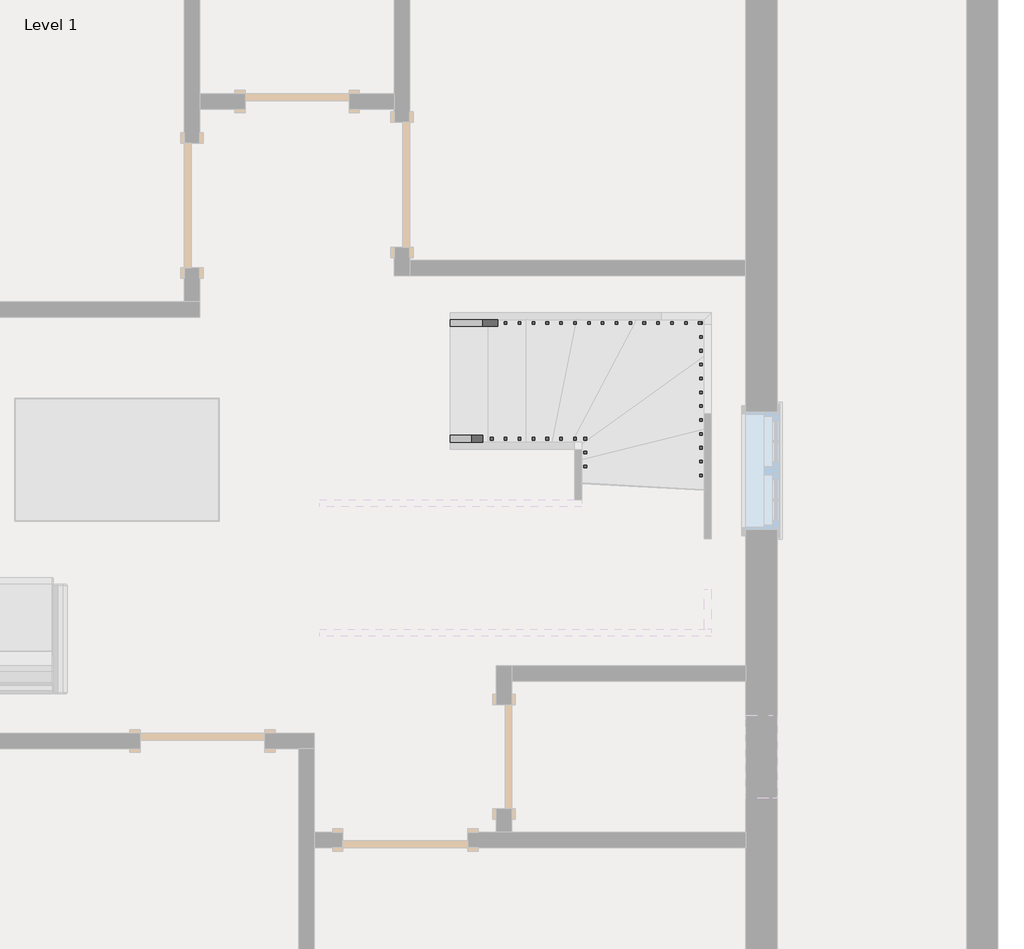
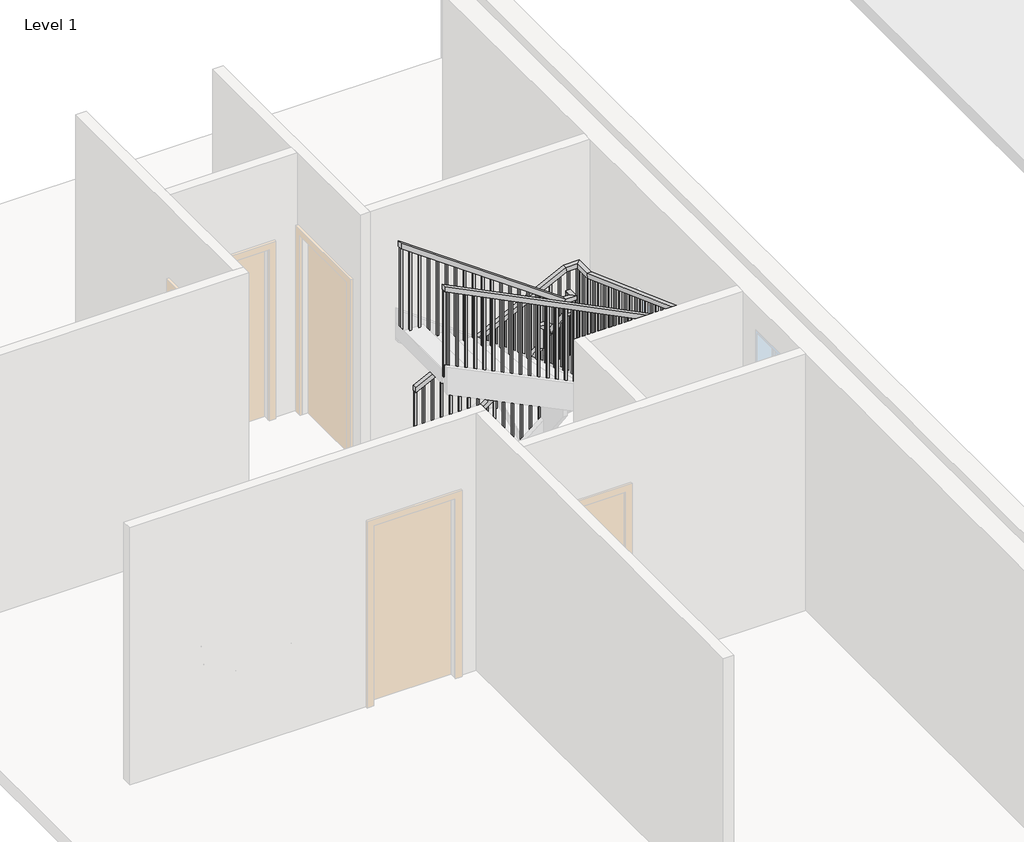
# One storey, part 2 of 3: 2 railings.
"""IFC4 building model written with IfcOpenShell, lengths in millimetres."""

from ifc_helpers import new_model, si_unit, frame, origin, place, context, project, spatial, polyline, outline, extrude, faceted_brep, element, save

model = new_model("IFC4")

# Units and contexts
model_context = context("Model", 3, world=origin())
ifc_project = project(units=[si_unit("LENGTHUNIT", "METRE", prefix="MILLI")], contexts=[model_context])

# Site, building, storey
site = spatial("IfcSite", under=ifc_project)
building = spatial("IfcBuilding", under=site)
storey = spatial("IfcBuildingStorey", under=building, Name="Level 1", Elevation=0.0)

# Railings
placement = place(None, origin())
element("IfcRailing", 1, ObjectType="Handrail - Rectangular", at=placement, inside=storey, context=model_context, shape_type="SolidModel", body=[
    faceted_brep([(158.6923968, 2074.8935985, 1083.7333333), (158.6923968, 2074.8935985, 1020.0053174), (158.6923968, 2024.0935985, 1020.0053174), (158.6923968, 2024.0935985, 1083.7333333), (1047.1901835, 2074.8935985, 1756.732376), (1097.9901835, 2074.8935985, 1731.4831856), (1097.9901835, 2024.0935985, 1731.4831856), (1047.1901835, 2024.0935985, 1756.732376), (1047.1901835, 2074.8935985, 2011.0303182), (1097.9901835, 2074.8935985, 1960.2303182), (1097.9901835, 2024.0935985, 1960.2303182), (1047.1901835, 2024.0935985, 2011.0303182), (1174.1901835, 2074.8935985, 2011.0303182), (1174.1901835, 2074.8935985, 1960.2303182), (1123.3901835, 2024.0935985, 1960.2303182), (1123.3901835, 2024.0935985, 2011.0303182), (1174.1901835, 1947.8935985, 2011.0303182), (1174.1901835, 1922.7437783, 1960.2303182), (1123.3901835, 1922.7437783, 1960.2303182), (1123.3901835, 1947.8935985, 2011.0303182), (1174.1901835, 1627.4476133, 2431.33697), (1174.1901835, 1576.6476133, 2414.1805221), (1123.3901835, 1576.6476133, 2414.1805221), (1123.3901835, 1627.4476133, 2431.33697), (1174.1901835, 1627.4476133, 2652.5821578), (1174.1901835, 1576.6476133, 2601.7821578), (1123.3901835, 1576.6476133, 2601.7821578), (1123.3901835, 1627.4476133, 2652.5821578), (1174.1901835, 1500.4476133, 2652.5821578), (1174.1901835, 1500.4476133, 2601.7821578), (1123.3901835, 1551.2476133, 2601.7821578), (1123.3901835, 1551.2476133, 2652.5821578), (1047.1901835, 1500.4476133, 2652.5821578), (1030.9951821, 1500.4476133, 2601.7821578), (1030.9951821, 1551.2476133, 2601.7821578), (1047.1901835, 1551.2476133, 2652.5821578), (-798.3242294, 1500.4476133, 3962.4), (-798.3242294, 1551.2476133, 3962.4), (-798.3242294, 1551.2476133, 3900.1059138), (-798.3242294, 1500.4476133, 3900.1059138)], [[[0, 1, 2, 3]], [[1, 0, 4, 5]], [[2, 1, 5, 6]], [[3, 2, 6, 7]], [[0, 3, 7, 4]], [[5, 4, 8, 9]], [[6, 5, 9, 10]], [[7, 6, 10, 11]], [[4, 7, 11, 8]], [[9, 8, 12, 13]], [[10, 9, 13, 14]], [[11, 10, 14, 15]], [[8, 11, 15, 12]], [[13, 12, 16, 17]], [[14, 13, 17, 18]], [[15, 14, 18, 19]], [[12, 15, 19, 16]], [[17, 16, 20, 21]], [[18, 17, 21, 22]], [[19, 18, 22, 23]], [[16, 19, 23, 20]], [[21, 20, 24, 25]], [[22, 21, 25, 26]], [[23, 22, 26, 27]], [[20, 23, 27, 24]], [[25, 24, 28, 29]], [[26, 25, 29, 30]], [[27, 26, 30, 31]], [[24, 27, 31, 28]], [[29, 28, 32, 33]], [[30, 29, 33, 34]], [[31, 30, 34, 35]], [[28, 31, 35, 32]], [[36, 37, 38, 39]], [[33, 32, 36, 39]], [[34, 33, 39, 38]], [[35, 34, 38, 37]], [[32, 35, 37, 36]]]),
    extrude(outline(polyline([(3881.4830025, -772.0848165), (3895.0033683, -791.1348165), (2878.6666667, -791.1348165), (2878.6666667, -772.0848165), (3881.4830025, -772.0848165)])), frame((0.0, 1516.3226133, 0.0), z_axis=(0.0, 1.0, 0.0), x_axis=(0.0, 0.0, 1.0)), (0.0, 0.0, 1.0), 19.05),
    extrude(outline(polyline([(3809.3743851, -670.4848165), (3822.8947509, -689.5348165), (2878.6666667, -689.5348165), (2878.6666667, -670.4848165), (3809.3743851, -670.4848165)])), frame((0.0, 1516.3226133, 0.0), z_axis=(0.0, 1.0, 0.0), x_axis=(0.0, 0.0, 1.0)), (0.0, 0.0, 1.0), 19.05),
    extrude(outline(polyline([(3737.2657677, -568.8848165), (3750.7861334, -587.9348165), (2878.6666667, -587.9348165), (2878.6666667, -568.8848165), (3737.2657677, -568.8848165)])), frame((0.0, 1516.3226133, 0.0), z_axis=(0.0, 1.0, 0.0), x_axis=(0.0, 0.0, 1.0)), (0.0, 0.0, 1.0), 19.05),
    extrude(outline(polyline([(3665.1571502, -467.2848165), (3678.677516, -486.3348165), (2709.3333333, -486.3348165), (2709.3333333, -467.2848165), (3665.1571502, -467.2848165)])), frame((0.0, 1516.3226133, 0.0), z_axis=(0.0, 1.0, 0.0), x_axis=(0.0, 0.0, 1.0)), (0.0, 0.0, 1.0), 19.05),
    extrude(outline(polyline([(3593.0485328, -365.6848165), (3606.5688986, -384.7348165), (2709.3333333, -384.7348165), (2709.3333333, -365.6848165), (3593.0485328, -365.6848165)])), frame((0.0, 1516.3226133, 0.0), z_axis=(0.0, 1.0, 0.0), x_axis=(0.0, 0.0, 1.0)), (0.0, 0.0, 1.0), 19.05),
    extrude(outline(polyline([(3520.9399154, -264.0848165), (3534.4602811, -283.1348165), (2709.3333333, -283.1348165), (2709.3333333, -264.0848165), (3520.9399154, -264.0848165)])), frame((0.0, 1516.3226133, 0.0), z_axis=(0.0, 1.0, 0.0), x_axis=(0.0, 0.0, 1.0)), (0.0, 0.0, 1.0), 19.05),
    extrude(outline(polyline([(3448.8312979, -162.4848165), (3462.3516637, -181.5348165), (2540.0, -181.5348165), (2540.0, -162.4848165), (3448.8312979, -162.4848165)])), frame((0.0, 1516.3226133, 0.0), z_axis=(0.0, 1.0, 0.0), x_axis=(0.0, 0.0, 1.0)), (0.0, 0.0, 1.0), 19.05),
    extrude(outline(polyline([(3376.7226805, -60.8848165), (3390.2430462, -79.9348165), (2540.0, -79.9348165), (2540.0, -60.8848165), (3376.7226805, -60.8848165)])), frame((0.0, 1516.3226133, 0.0), z_axis=(0.0, 1.0, 0.0), x_axis=(0.0, 0.0, 1.0)), (0.0, 0.0, 1.0), 19.05),
    extrude(outline(polyline([(3304.614063, 40.7151835), (3318.1344288, 21.6651835), (2370.6666667, 21.6651835), (2370.6666667, 40.7151835), (3304.614063, 40.7151835)])), frame((0.0, 1516.3226133, 0.0), z_axis=(0.0, 1.0, 0.0), x_axis=(0.0, 0.0, 1.0)), (0.0, 0.0, 1.0), 19.05),
    extrude(outline(polyline([(3232.5054456, 142.3151835), (3246.0258114, 123.2651835), (2370.6666667, 123.2651835), (2370.6666667, 142.3151835), (3232.5054456, 142.3151835)])), frame((0.0, 1516.3226133, 0.0), z_axis=(0.0, 1.0, 0.0), x_axis=(0.0, 0.0, 1.0)), (0.0, 0.0, 1.0), 19.05),
    extrude(outline(polyline([(3160.3968282, 243.9151835), (3173.9171939, 224.8651835), (2370.6666667, 224.8651835), (2370.6666667, 243.9151835), (3160.3968282, 243.9151835)])), frame((0.0, 1516.3226133, 0.0), z_axis=(0.0, 1.0, 0.0), x_axis=(0.0, 0.0, 1.0)), (0.0, 0.0, 1.0), 19.05),
    extrude(outline(polyline([(3088.2882107, 345.5151835), (3101.8085765, 326.4651835), (2201.3333333, 326.4651835), (2201.3333333, 345.5151835), (3088.2882107, 345.5151835)])), frame((0.0, 1516.3226133, 0.0), z_axis=(0.0, 1.0, 0.0), x_axis=(0.0, 0.0, 1.0)), (0.0, 0.0, 1.0), 19.05),
    extrude(outline(polyline([(3016.1795933, 447.1151835), (3029.6999591, 428.0651835), (2201.3333333, 428.0651835), (2201.3333333, 447.1151835), (3016.1795933, 447.1151835)])), frame((0.0, 1516.3226133, 0.0), z_axis=(0.0, 1.0, 0.0), x_axis=(0.0, 0.0, 1.0)), (0.0, 0.0, 1.0), 19.05),
    extrude(outline(polyline([(2944.0709758, 548.7151835), (2957.5913416, 529.6651835), (2032.0, 529.6651835), (2032.0, 548.7151835), (2944.0709758, 548.7151835)])), frame((0.0, 1516.3226133, 0.0), z_axis=(0.0, 1.0, 0.0), x_axis=(0.0, 0.0, 1.0)), (0.0, 0.0, 1.0), 19.05),
    extrude(outline(polyline([(2871.9623584, 650.3151835), (2885.4827242, 631.2651835), (2032.0, 631.2651835), (2032.0, 650.3151835), (2871.9623584, 650.3151835)])), frame((0.0, 1516.3226133, 0.0), z_axis=(0.0, 1.0, 0.0), x_axis=(0.0, 0.0, 1.0)), (0.0, 0.0, 1.0), 19.05),
    extrude(outline(polyline([(2799.853741, 751.9151835), (2813.3741067, 732.8651835), (2032.0, 732.8651835), (2032.0, 751.9151835), (2799.853741, 751.9151835)])), frame((0.0, 1516.3226133, 0.0), z_axis=(0.0, 1.0, 0.0), x_axis=(0.0, 0.0, 1.0)), (0.0, 0.0, 1.0), 19.05),
    extrude(outline(polyline([(2727.7451235, 853.5151835), (2741.2654893, 834.4651835), (1862.6666667, 834.4651835), (1862.6666667, 853.5151835), (2727.7451235, 853.5151835)])), frame((0.0, 1516.3226133, 0.0), z_axis=(0.0, 1.0, 0.0), x_axis=(0.0, 0.0, 1.0)), (0.0, 0.0, 1.0), 19.05),
    extrude(outline(polyline([(2655.6365061, 955.1151835), (2669.1568719, 936.0651835), (1862.6666667, 936.0651835), (1862.6666667, 955.1151835), (2655.6365061, 955.1151835)])), frame((0.0, 1516.3226133, 0.0), z_axis=(0.0, 1.0, 0.0), x_axis=(0.0, 0.0, 1.0)), (0.0, 0.0, 1.0), 19.05),
    extrude(outline(polyline([(2583.5278887, 1056.7151835), (2597.0482544, 1037.6651835), (1693.3333333, 1037.6651835), (1693.3333333, 1056.7151835), (2583.5278887, 1056.7151835)])), frame((0.0, 1516.3226133, 0.0), z_axis=(0.0, 1.0, 0.0), x_axis=(0.0, 0.0, 1.0)), (0.0, 0.0, 1.0), 19.05),
    extrude(outline(polyline([(1139.2651835, 1551.0185985), (1158.3151835, 1551.0185985), (1158.3151835, 1531.9685985), (1139.2651835, 1531.9685985), (1139.2651835, 1551.0185985)])), frame((0.0, 0.0, 1524.0), z_axis=(0.0, 0.0, 1.0), x_axis=(1.0, 0.0, 0.0)), (0.0, 0.0, 1.0), 1077.7821578),
    extrude(outline(polyline([(1633.5685985, 2339.5212353), (1652.6185985, 2314.5346787), (1652.6185985, 1354.6666667), (1633.5685985, 1354.6666667), (1633.5685985, 2339.5212353)])), frame((1139.2651835, 0.0, 0.0), z_axis=(1.0, 0.0, 0.0), x_axis=(0.0, 1.0, 0.0)), (0.0, 0.0, 1.0), 19.05),
    extrude(outline(polyline([(1735.1685985, 2206.2596006), (1754.2185985, 2181.273044), (1754.2185985, 1354.6666667), (1735.1685985, 1354.6666667), (1735.1685985, 2206.2596006)])), frame((1139.2651835, 0.0, 0.0), z_axis=(1.0, 0.0, 0.0), x_axis=(0.0, 1.0, 0.0)), (0.0, 0.0, 1.0), 19.05),
    extrude(outline(polyline([(1836.7685985, 2072.9979659), (1855.8185985, 2048.0114093), (1855.8185985, 1185.3333333), (1836.7685985, 1185.3333333), (1836.7685985, 2072.9979659)])), frame((1139.2651835, 0.0, 0.0), z_axis=(1.0, 0.0, 0.0), x_axis=(0.0, 1.0, 0.0)), (0.0, 0.0, 1.0), 19.05),
    extrude(outline(polyline([(1938.3685985, 1939.7363312), (1957.4185985, 1914.7497746), (1957.4185985, 1016.0), (1938.3685985, 1016.0), (1938.3685985, 1939.7363312)])), frame((1139.2651835, 0.0, 0.0), z_axis=(1.0, 0.0, 0.0), x_axis=(0.0, 1.0, 0.0)), (0.0, 0.0, 1.0), 19.05),
    extrude(outline(polyline([(1063.5673968, 2039.9685985), (1063.5673968, 2059.0185985), (1082.6173968, 2059.0185985), (1082.6173968, 2039.9685985), (1063.5673968, 2039.9685985)])), frame((0.0, 0.0, 846.6666667), z_axis=(0.0, 0.0, 1.0), x_axis=(1.0, 0.0, 0.0)), (0.0, 0.0, 1.0), 1113.5636515),
    extrude(outline(polyline([(1642.8813066, 981.0173968), (1628.451747, 961.9673968), (677.3333333, 961.9673968), (677.3333333, 981.0173968), (1642.8813066, 981.0173968)])), frame((0.0, 2039.9685985, 0.0), z_axis=(0.0, 1.0, 0.0), x_axis=(0.0, 0.0, 1.0)), (0.0, 0.0, 1.0), 19.05),
    extrude(outline(polyline([(1565.9236554, 879.4173968), (1551.4940958, 860.3673968), (508.0, 860.3673968), (508.0, 879.4173968), (1565.9236554, 879.4173968)])), frame((0.0, 2039.9685985, 0.0), z_axis=(0.0, 1.0, 0.0), x_axis=(0.0, 0.0, 1.0)), (0.0, 0.0, 1.0), 19.05),
    extrude(outline(polyline([(1488.9660042, 777.8173968), (1474.5364446, 758.7673968), (508.0, 758.7673968), (508.0, 777.8173968), (1488.9660042, 777.8173968)])), frame((0.0, 2039.9685985, 0.0), z_axis=(0.0, 1.0, 0.0), x_axis=(0.0, 0.0, 1.0)), (0.0, 0.0, 1.0), 19.05),
    extrude(outline(polyline([(1412.008353, 676.2173968), (1397.5787934, 657.1673968), (338.6666667, 657.1673968), (338.6666667, 676.2173968), (1412.008353, 676.2173968)])), frame((0.0, 2039.9685985, 0.0), z_axis=(0.0, 1.0, 0.0), x_axis=(0.0, 0.0, 1.0)), (0.0, 0.0, 1.0), 19.05),
    extrude(outline(polyline([(1335.0507019, 574.6173968), (1320.6211423, 555.5673968), (338.6666667, 555.5673968), (338.6666667, 574.6173968), (1335.0507019, 574.6173968)])), frame((0.0, 2039.9685985, 0.0), z_axis=(0.0, 1.0, 0.0), x_axis=(0.0, 0.0, 1.0)), (0.0, 0.0, 1.0), 19.05),
    extrude(outline(polyline([(1258.0930507, 473.0173968), (1243.6634911, 453.9673968), (338.6666667, 453.9673968), (338.6666667, 473.0173968), (1258.0930507, 473.0173968)])), frame((0.0, 2039.9685985, 0.0), z_axis=(0.0, 1.0, 0.0), x_axis=(0.0, 0.0, 1.0)), (0.0, 0.0, 1.0), 19.05),
    extrude(outline(polyline([(1181.1353995, 371.4173968), (1166.7058399, 352.3673968), (169.3333333, 352.3673968), (169.3333333, 371.4173968), (1181.1353995, 371.4173968)])), frame((0.0, 2039.9685985, 0.0), z_axis=(0.0, 1.0, 0.0), x_axis=(0.0, 0.0, 1.0)), (0.0, 0.0, 1.0), 19.05),
    extrude(outline(polyline([(1104.1777483, 269.8173968), (1089.7481887, 250.7673968), (169.3333333, 250.7673968), (169.3333333, 269.8173968), (1104.1777483, 269.8173968)])), frame((0.0, 2039.9685985, 0.0), z_axis=(0.0, 1.0, 0.0), x_axis=(0.0, 0.0, 1.0)), (0.0, 0.0, 1.0), 19.05),
    extrude(outline(polyline([(1139.2651835, 1535.3726133), (1158.3151835, 1535.3726133), (1158.3151835, 1516.3226133), (1139.2651835, 1516.3226133), (1139.2651835, 1535.3726133)])), frame((0.0, 0.0, 1524.0), z_axis=(0.0, 0.0, 1.0), x_axis=(1.0, 0.0, 0.0)), (0.0, 0.0, 1.0), 1077.7821578),
    extrude(outline(polyline([(1139.2651835, 2039.9685985), (1139.2651835, 2059.0185985), (1158.3151835, 2059.0185985), (1158.3151835, 2039.9685985), (1139.2651835, 2039.9685985)])), frame((0.0, 0.0, 846.6666667), z_axis=(0.0, 0.0, 1.0), x_axis=(1.0, 0.0, 0.0)), (0.0, 0.0, 1.0), 1113.5636515),
    extrude(outline(polyline([(3886.585548, -779.2742294), (3900.1059138, -798.3242294), (2878.6666667, -798.3242294), (2878.6666667, -779.2742294), (3886.585548, -779.2742294)])), frame((0.0, 1516.3226133, 0.0), z_axis=(0.0, 1.0, 0.0), x_axis=(0.0, 0.0, 1.0)), (0.0, 0.0, 1.0), 19.05),
    extrude(outline(polyline([(1034.434877, 177.7423968), (1020.0053174, 158.6923968), (169.3333333, 158.6923968), (169.3333333, 177.7423968), (1034.434877, 177.7423968)])), frame((0.0, 2039.9685985, 0.0), z_axis=(0.0, 1.0, 0.0), x_axis=(0.0, 0.0, 1.0)), (0.0, 0.0, 1.0), 19.05),
])
element("IfcRailing", 2, ObjectType="Handrail - Rectangular", at=placement, inside=storey, context=model_context, shape_type="SolidModel", body=[
    faceted_brep([(158.6923968, 2922.8476133, 1083.7333333), (158.6923968, 2922.8476133, 1027.0325724), (158.6923968, 2872.0476133, 1027.0325724), (158.6923968, 2872.0476133, 1083.7333333), (1841.0143863, 2922.8476133, 1917.8084972), (1852.9161672, 2922.8476133, 1867.0084972), (1852.9161672, 2872.0476133, 1867.0084972), (1841.0143863, 2872.0476133, 1917.8084972), (2022.1441983, 2922.8476133, 1917.8084972), (2022.1441983, 2922.8476133, 1867.0084972), (1971.3441983, 2872.0476133, 1867.0084972), (1971.3441983, 2872.0476133, 1917.8084972), (2022.1441983, 2686.7050655, 1917.8084972), (2022.1441983, 2677.692274, 1867.0084972), (1971.3441983, 2677.692274, 1867.0084972), (1971.3441983, 2686.7050655, 1917.8084972), (2022.1441983, 796.951655, 2610.1505936), (2022.1441983, 787.9388635, 2559.3505936), (1971.3441983, 787.9388635, 2559.3505936), (1971.3441983, 796.951655, 2610.1505936), (2022.1441983, 652.4935985, 2610.1505936), (2022.1441983, 652.4935985, 2559.3505936), (1971.3441983, 703.2935985, 2559.3505936), (1971.3441983, 703.2935985, 2610.1505936), (1909.402346, 652.4935985, 2610.1505936), (1897.4228813, 652.4935985, 2559.3505936), (1897.4228813, 703.2935985, 2559.3505936), (1909.402346, 703.2935985, 2610.1505936), (-798.3242294, 652.4935985, 3962.4), (-798.3242294, 703.2935985, 3962.4), (-798.3242294, 703.2935985, 3905.6174077), (-798.3242294, 652.4935985, 3905.6174077)], [[[0, 1, 2, 3]], [[1, 0, 4, 5]], [[2, 1, 5, 6]], [[3, 2, 6, 7]], [[0, 3, 7, 4]], [[5, 4, 8, 9]], [[6, 5, 9, 10]], [[7, 6, 10, 11]], [[4, 7, 11, 8]], [[9, 8, 12, 13]], [[10, 9, 13, 14]], [[11, 10, 14, 15]], [[8, 11, 15, 12]], [[13, 12, 16, 17]], [[14, 13, 17, 18]], [[15, 14, 18, 19]], [[12, 15, 19, 16]], [[17, 16, 20, 21]], [[18, 17, 21, 22]], [[19, 18, 22, 23]], [[16, 19, 23, 20]], [[21, 20, 24, 25]], [[22, 21, 25, 26]], [[23, 22, 26, 27]], [[20, 23, 27, 24]], [[28, 29, 30, 31]], [[25, 24, 28, 31]], [[26, 25, 31, 30]], [[27, 26, 30, 29]], [[24, 27, 29, 28]]]),
    extrude(outline(polyline([(3884.4709318, -755.9808017), (2878.6666667, -755.9808017), (2878.6666667, -736.9308017), (3874.9572862, -736.9308017), (3884.4709318, -755.9808017)])), frame((0.0, 668.3685985, 0.0), z_axis=(0.0, 1.0, 0.0), x_axis=(0.0, 0.0, 1.0)), (0.0, 0.0, 1.0), 19.05),
    extrude(outline(polyline([(3833.7314883, -654.3808017), (2878.6666667, -654.3808017), (2878.6666667, -635.3308017), (3824.2178426, -635.3308017), (3833.7314883, -654.3808017)])), frame((0.0, 668.3685985, 0.0), z_axis=(0.0, 1.0, 0.0), x_axis=(0.0, 0.0, 1.0)), (0.0, 0.0, 1.0), 19.05),
    extrude(outline(polyline([(3782.9920447, -552.7808017), (2878.6666667, -552.7808017), (2878.6666667, -533.7308017), (3773.4783991, -533.7308017), (3782.9920447, -552.7808017)])), frame((0.0, 668.3685985, 0.0), z_axis=(0.0, 1.0, 0.0), x_axis=(0.0, 0.0, 1.0)), (0.0, 0.0, 1.0), 19.05),
    extrude(outline(polyline([(3732.2526012, -451.1808017), (2709.3333333, -451.1808017), (2709.3333333, -432.1308017), (3722.7389555, -432.1308017), (3732.2526012, -451.1808017)])), frame((0.0, 668.3685985, 0.0), z_axis=(0.0, 1.0, 0.0), x_axis=(0.0, 0.0, 1.0)), (0.0, 0.0, 1.0), 19.05),
    extrude(outline(polyline([(3681.5131577, -349.5808017), (2709.3333333, -349.5808017), (2709.3333333, -330.5308017), (3671.999512, -330.5308017), (3681.5131577, -349.5808017)])), frame((0.0, 668.3685985, 0.0), z_axis=(0.0, 1.0, 0.0), x_axis=(0.0, 0.0, 1.0)), (0.0, 0.0, 1.0), 19.05),
    extrude(outline(polyline([(3630.7737141, -247.9808017), (2540.0, -247.9808017), (2540.0, -228.9308017), (3621.2600685, -228.9308017), (3630.7737141, -247.9808017)])), frame((0.0, 668.3685985, 0.0), z_axis=(0.0, 1.0, 0.0), x_axis=(0.0, 0.0, 1.0)), (0.0, 0.0, 1.0), 19.05),
    extrude(outline(polyline([(3580.0342706, -146.3808017), (2540.0, -146.3808017), (2540.0, -127.3308017), (3570.5206249, -127.3308017), (3580.0342706, -146.3808017)])), frame((0.0, 668.3685985, 0.0), z_axis=(0.0, 1.0, 0.0), x_axis=(0.0, 0.0, 1.0)), (0.0, 0.0, 1.0), 19.05),
    extrude(outline(polyline([(3529.294827, -44.7808017), (2540.0, -44.7808017), (2540.0, -25.7308017), (3519.7811814, -25.7308017), (3529.294827, -44.7808017)])), frame((0.0, 668.3685985, 0.0), z_axis=(0.0, 1.0, 0.0), x_axis=(0.0, 0.0, 1.0)), (0.0, 0.0, 1.0), 19.05),
    extrude(outline(polyline([(3478.5553835, 56.8191983), (2370.6666667, 56.8191983), (2370.6666667, 75.8691983), (3469.0417378, 75.8691983), (3478.5553835, 56.8191983)])), frame((0.0, 668.3685985, 0.0), z_axis=(0.0, 1.0, 0.0), x_axis=(0.0, 0.0, 1.0)), (0.0, 0.0, 1.0), 19.05),
    extrude(outline(polyline([(3427.81594, 158.4191983), (2370.6666667, 158.4191983), (2370.6666667, 177.4691983), (3418.3022943, 177.4691983), (3427.81594, 158.4191983)])), frame((0.0, 668.3685985, 0.0), z_axis=(0.0, 1.0, 0.0), x_axis=(0.0, 0.0, 1.0)), (0.0, 0.0, 1.0), 19.05),
    extrude(outline(polyline([(3377.0764964, 260.0191983), (2370.6666667, 260.0191983), (2370.6666667, 279.0691983), (3367.5628508, 279.0691983), (3377.0764964, 260.0191983)])), frame((0.0, 668.3685985, 0.0), z_axis=(0.0, 1.0, 0.0), x_axis=(0.0, 0.0, 1.0)), (0.0, 0.0, 1.0), 19.05),
    extrude(outline(polyline([(3326.3370529, 361.6191983), (2201.3333333, 361.6191983), (2201.3333333, 380.6691983), (3316.8234072, 380.6691983), (3326.3370529, 361.6191983)])), frame((0.0, 668.3685985, 0.0), z_axis=(0.0, 1.0, 0.0), x_axis=(0.0, 0.0, 1.0)), (0.0, 0.0, 1.0), 19.05),
    extrude(outline(polyline([(3275.5976093, 463.2191983), (2201.3333333, 463.2191983), (2201.3333333, 482.2691983), (3266.0839637, 482.2691983), (3275.5976093, 463.2191983)])), frame((0.0, 668.3685985, 0.0), z_axis=(0.0, 1.0, 0.0), x_axis=(0.0, 0.0, 1.0)), (0.0, 0.0, 1.0), 19.05),
    extrude(outline(polyline([(3224.8581658, 564.8191983), (2201.3333333, 564.8191983), (2201.3333333, 583.8691983), (3215.3445201, 583.8691983), (3224.8581658, 564.8191983)])), frame((0.0, 668.3685985, 0.0), z_axis=(0.0, 1.0, 0.0), x_axis=(0.0, 0.0, 1.0)), (0.0, 0.0, 1.0), 19.05),
    extrude(outline(polyline([(3174.1187223, 666.4191983), (2032.0, 666.4191983), (2032.0, 685.4691983), (3164.6050766, 685.4691983), (3174.1187223, 666.4191983)])), frame((0.0, 668.3685985, 0.0), z_axis=(0.0, 1.0, 0.0), x_axis=(0.0, 0.0, 1.0)), (0.0, 0.0, 1.0), 19.05),
    extrude(outline(polyline([(3123.3792787, 768.0191983), (2032.0, 768.0191983), (2032.0, 787.0691983), (3113.865633, 787.0691983), (3123.3792787, 768.0191983)])), frame((0.0, 668.3685985, 0.0), z_axis=(0.0, 1.0, 0.0), x_axis=(0.0, 0.0, 1.0)), (0.0, 0.0, 1.0), 19.05),
    extrude(outline(polyline([(3072.6398352, 869.6191983), (2032.0, 869.6191983), (2032.0, 888.6691983), (3063.1261895, 888.6691983), (3072.6398352, 869.6191983)])), frame((0.0, 668.3685985, 0.0), z_axis=(0.0, 1.0, 0.0), x_axis=(0.0, 0.0, 1.0)), (0.0, 0.0, 1.0), 19.05),
    extrude(outline(polyline([(3021.9003916, 971.2191983), (2032.0, 971.2191983), (2032.0, 990.2691983), (3012.386746, 990.2691983), (3021.9003916, 971.2191983)])), frame((0.0, 668.3685985, 0.0), z_axis=(0.0, 1.0, 0.0), x_axis=(0.0, 0.0, 1.0)), (0.0, 0.0, 1.0), 19.05),
    extrude(outline(polyline([(2971.1609481, 1072.8191983), (1862.6666667, 1072.8191983), (1862.6666667, 1091.8691983), (2961.6473024, 1091.8691983), (2971.1609481, 1072.8191983)])), frame((0.0, 668.3685985, 0.0), z_axis=(0.0, 1.0, 0.0), x_axis=(0.0, 0.0, 1.0)), (0.0, 0.0, 1.0), 19.05),
    extrude(outline(polyline([(2920.4215046, 1174.4191983), (1862.6666667, 1174.4191983), (1862.6666667, 1193.4691983), (2910.9078589, 1193.4691983), (2920.4215046, 1174.4191983)])), frame((0.0, 668.3685985, 0.0), z_axis=(0.0, 1.0, 0.0), x_axis=(0.0, 0.0, 1.0)), (0.0, 0.0, 1.0), 19.05),
    extrude(outline(polyline([(2869.682061, 1276.0191983), (1862.6666667, 1276.0191983), (1862.6666667, 1295.0691983), (2860.1684153, 1295.0691983), (2869.682061, 1276.0191983)])), frame((0.0, 668.3685985, 0.0), z_axis=(0.0, 1.0, 0.0), x_axis=(0.0, 0.0, 1.0)), (0.0, 0.0, 1.0), 19.05),
    extrude(outline(polyline([(2818.9426175, 1377.6191983), (1693.3333333, 1377.6191983), (1693.3333333, 1396.6691983), (2809.4289718, 1396.6691983), (2818.9426175, 1377.6191983)])), frame((0.0, 668.3685985, 0.0), z_axis=(0.0, 1.0, 0.0), x_axis=(0.0, 0.0, 1.0)), (0.0, 0.0, 1.0), 19.05),
    extrude(outline(polyline([(2768.2031739, 1479.2191983), (1693.3333333, 1479.2191983), (1693.3333333, 1498.2691983), (2758.6895283, 1498.2691983), (2768.2031739, 1479.2191983)])), frame((0.0, 668.3685985, 0.0), z_axis=(0.0, 1.0, 0.0), x_axis=(0.0, 0.0, 1.0)), (0.0, 0.0, 1.0), 19.05),
    extrude(outline(polyline([(2717.4637304, 1580.8191983), (1693.3333333, 1580.8191983), (1693.3333333, 1599.8691983), (2707.9500847, 1599.8691983), (2717.4637304, 1580.8191983)])), frame((0.0, 668.3685985, 0.0), z_axis=(0.0, 1.0, 0.0), x_axis=(0.0, 0.0, 1.0)), (0.0, 0.0, 1.0), 19.05),
    extrude(outline(polyline([(2666.7242869, 1682.4191983), (1693.3333333, 1682.4191983), (1693.3333333, 1701.4691983), (2657.2106412, 1701.4691983), (2666.7242869, 1682.4191983)])), frame((0.0, 668.3685985, 0.0), z_axis=(0.0, 1.0, 0.0), x_axis=(0.0, 0.0, 1.0)), (0.0, 0.0, 1.0), 19.05),
    extrude(outline(polyline([(2615.9848433, 1784.0191983), (1693.3333333, 1784.0191983), (1693.3333333, 1803.0691983), (2606.4711976, 1803.0691983), (2615.9848433, 1784.0191983)])), frame((0.0, 668.3685985, 0.0), z_axis=(0.0, 1.0, 0.0), x_axis=(0.0, 0.0, 1.0)), (0.0, 0.0, 1.0), 19.05),
    extrude(outline(polyline([(2565.2453998, 1885.6191983), (1524.0, 1885.6191983), (1524.0, 1904.6691983), (2555.7317541, 1904.6691983), (2565.2453998, 1885.6191983)])), frame((0.0, 668.3685985, 0.0), z_axis=(0.0, 1.0, 0.0), x_axis=(0.0, 0.0, 1.0)), (0.0, 0.0, 1.0), 19.05),
    extrude(outline(polyline([(2006.2691983, 773.3726133), (2006.2691983, 754.3226133), (1987.2191983, 754.3226133), (1987.2191983, 773.3726133), (2006.2691983, 773.3726133)])), frame((0.0, 0.0, 1524.0), z_axis=(0.0, 0.0, 1.0), x_axis=(1.0, 0.0, 0.0)), (0.0, 0.0, 1.0), 1035.3505936),
    extrude(outline(polyline([(874.9726133, 2527.4643546), (874.9726133, 1524.0), (855.9226133, 1524.0), (855.9226133, 2534.443634), (874.9726133, 2527.4643546)])), frame((1987.2191983, 0.0, 0.0), z_axis=(1.0, 0.0, 0.0), x_axis=(0.0, 1.0, 0.0)), (0.0, 0.0, 1.0), 19.05),
    extrude(outline(polyline([(976.5726133, 2490.2415315), (976.5726133, 1524.0), (957.5226133, 1524.0), (957.5226133, 2497.2208108), (976.5726133, 2490.2415315)])), frame((1987.2191983, 0.0, 0.0), z_axis=(1.0, 0.0, 0.0), x_axis=(0.0, 1.0, 0.0)), (0.0, 0.0, 1.0), 19.05),
    extrude(outline(polyline([(1078.1726133, 2453.0187083), (1078.1726133, 1524.0), (1059.1226133, 1524.0), (1059.1226133, 2459.9979877), (1078.1726133, 2453.0187083)])), frame((1987.2191983, 0.0, 0.0), z_axis=(1.0, 0.0, 0.0), x_axis=(0.0, 1.0, 0.0)), (0.0, 0.0, 1.0), 19.05),
    extrude(outline(polyline([(1179.7726133, 2415.7958852), (1179.7726133, 1524.0), (1160.7226133, 1524.0), (1160.7226133, 2422.7751645), (1179.7726133, 2415.7958852)])), frame((1987.2191983, 0.0, 0.0), z_axis=(1.0, 0.0, 0.0), x_axis=(0.0, 1.0, 0.0)), (0.0, 0.0, 1.0), 19.05),
    extrude(outline(polyline([(1281.3726133, 2378.573062), (1281.3726133, 1524.0), (1262.3226133, 1524.0), (1262.3226133, 2385.5523414), (1281.3726133, 2378.573062)])), frame((1987.2191983, 0.0, 0.0), z_axis=(1.0, 0.0, 0.0), x_axis=(0.0, 1.0, 0.0)), (0.0, 0.0, 1.0), 19.05),
    extrude(outline(polyline([(1382.9726133, 2341.3502389), (1382.9726133, 1354.6666667), (1363.9226133, 1354.6666667), (1363.9226133, 2348.3295182), (1382.9726133, 2341.3502389)])), frame((1987.2191983, 0.0, 0.0), z_axis=(1.0, 0.0, 0.0), x_axis=(0.0, 1.0, 0.0)), (0.0, 0.0, 1.0), 19.05),
    extrude(outline(polyline([(1484.5726133, 2304.1274157), (1484.5726133, 1354.6666667), (1465.5226133, 1354.6666667), (1465.5226133, 2311.1066951), (1484.5726133, 2304.1274157)])), frame((1987.2191983, 0.0, 0.0), z_axis=(1.0, 0.0, 0.0), x_axis=(0.0, 1.0, 0.0)), (0.0, 0.0, 1.0), 19.05),
    extrude(outline(polyline([(1586.1726133, 2266.9045926), (1586.1726133, 1354.6666667), (1567.1226133, 1354.6666667), (1567.1226133, 2273.8838719), (1586.1726133, 2266.9045926)])), frame((1987.2191983, 0.0, 0.0), z_axis=(1.0, 0.0, 0.0), x_axis=(0.0, 1.0, 0.0)), (0.0, 0.0, 1.0), 19.05),
    extrude(outline(polyline([(1687.7726133, 2229.6817694), (1687.7726133, 1354.6666667), (1668.7226133, 1354.6666667), (1668.7226133, 2236.6610488), (1687.7726133, 2229.6817694)])), frame((1987.2191983, 0.0, 0.0), z_axis=(1.0, 0.0, 0.0), x_axis=(0.0, 1.0, 0.0)), (0.0, 0.0, 1.0), 19.05),
    extrude(outline(polyline([(1789.3726133, 2192.4589463), (1789.3726133, 1185.3333333), (1770.3226133, 1185.3333333), (1770.3226133, 2199.4382256), (1789.3726133, 2192.4589463)])), frame((1987.2191983, 0.0, 0.0), z_axis=(1.0, 0.0, 0.0), x_axis=(0.0, 1.0, 0.0)), (0.0, 0.0, 1.0), 19.05),
    extrude(outline(polyline([(1890.9726133, 2155.2361231), (1890.9726133, 1185.3333333), (1871.9226133, 1185.3333333), (1871.9226133, 2162.2154025), (1890.9726133, 2155.2361231)])), frame((1987.2191983, 0.0, 0.0), z_axis=(1.0, 0.0, 0.0), x_axis=(0.0, 1.0, 0.0)), (0.0, 0.0, 1.0), 19.05),
    extrude(outline(polyline([(1992.5726133, 2118.0133), (1992.5726133, 1185.3333333), (1973.5226133, 1185.3333333), (1973.5226133, 2124.9925793), (1992.5726133, 2118.0133)])), frame((1987.2191983, 0.0, 0.0), z_axis=(1.0, 0.0, 0.0), x_axis=(0.0, 1.0, 0.0)), (0.0, 0.0, 1.0), 19.05),
    extrude(outline(polyline([(2094.1726133, 2080.7904769), (2094.1726133, 1185.3333333), (2075.1226133, 1185.3333333), (2075.1226133, 2087.7697562), (2094.1726133, 2080.7904769)])), frame((1987.2191983, 0.0, 0.0), z_axis=(1.0, 0.0, 0.0), x_axis=(0.0, 1.0, 0.0)), (0.0, 0.0, 1.0), 19.05),
    extrude(outline(polyline([(2195.7726133, 2043.5676537), (2195.7726133, 1016.0), (2176.7226133, 1016.0), (2176.7226133, 2050.546933), (2195.7726133, 2043.5676537)])), frame((1987.2191983, 0.0, 0.0), z_axis=(1.0, 0.0, 0.0), x_axis=(0.0, 1.0, 0.0)), (0.0, 0.0, 1.0), 19.05),
    extrude(outline(polyline([(2297.3726133, 2006.3448306), (2297.3726133, 1016.0), (2278.3226133, 1016.0), (2278.3226133, 2013.3241099), (2297.3726133, 2006.3448306)])), frame((1987.2191983, 0.0, 0.0), z_axis=(1.0, 0.0, 0.0), x_axis=(0.0, 1.0, 0.0)), (0.0, 0.0, 1.0), 19.05),
    extrude(outline(polyline([(2398.9726133, 1969.1220074), (2398.9726133, 1016.0), (2379.9226133, 1016.0), (2379.9226133, 1976.1012867), (2398.9726133, 1969.1220074)])), frame((1987.2191983, 0.0, 0.0), z_axis=(1.0, 0.0, 0.0), x_axis=(0.0, 1.0, 0.0)), (0.0, 0.0, 1.0), 19.05),
    extrude(outline(polyline([(2500.5726133, 1931.8991843), (2500.5726133, 1016.0), (2481.5226133, 1016.0), (2481.5226133, 1938.8784636), (2500.5726133, 1931.8991843)])), frame((1987.2191983, 0.0, 0.0), z_axis=(1.0, 0.0, 0.0), x_axis=(0.0, 1.0, 0.0)), (0.0, 0.0, 1.0), 19.05),
    extrude(outline(polyline([(2602.1726133, 1894.6763611), (2602.1726133, 1016.0), (2583.1226133, 1016.0), (2583.1226133, 1901.6556405), (2602.1726133, 1894.6763611)])), frame((1987.2191983, 0.0, 0.0), z_axis=(1.0, 0.0, 0.0), x_axis=(0.0, 1.0, 0.0)), (0.0, 0.0, 1.0), 19.05),
    extrude(outline(polyline([(2006.2691983, 2703.7726133), (2006.2691983, 2684.7226133), (1987.2191983, 2684.7226133), (1987.2191983, 2703.7726133), (2006.2691983, 2703.7726133)])), frame((0.0, 0.0, 846.6666667), z_axis=(0.0, 0.0, 1.0), x_axis=(1.0, 0.0, 0.0)), (0.0, 0.0, 1.0), 1020.3418305),
    extrude(outline(polyline([(2006.2691983, 2805.3726133), (2006.2691983, 2786.3226133), (1987.2191983, 2786.3226133), (1987.2191983, 2805.3726133), (2006.2691983, 2805.3726133)])), frame((0.0, 0.0, 846.6666667), z_axis=(0.0, 0.0, 1.0), x_axis=(1.0, 0.0, 0.0)), (0.0, 0.0, 1.0), 1020.3418305),
    extrude(outline(polyline([(1977.9673968, 2906.9726133), (1997.0173968, 2906.9726133), (1997.0173968, 2887.9226133), (1977.9673968, 2887.9226133), (1977.9673968, 2906.9726133)])), frame((0.0, 0.0, 846.6666667), z_axis=(0.0, 0.0, 1.0), x_axis=(1.0, 0.0, 0.0)), (0.0, 0.0, 1.0), 1020.3418305),
    extrude(outline(polyline([(1876.3673968, 2906.9726133), (1895.4173968, 2906.9726133), (1895.4173968, 2887.9226133), (1876.3673968, 2887.9226133), (1876.3673968, 2906.9726133)])), frame((0.0, 0.0, 846.6666667), z_axis=(0.0, 0.0, 1.0), x_axis=(1.0, 0.0, 0.0)), (0.0, 0.0, 1.0), 1020.3418305),
    extrude(outline(polyline([(1828.2632695, 1774.7673968), (846.6666667, 1774.7673968), (846.6666667, 1793.8173968), (1837.7080321, 1793.8173968), (1828.2632695, 1774.7673968)])), frame((0.0, 2887.9226133, 0.0), z_axis=(0.0, 1.0, 0.0), x_axis=(0.0, 0.0, 1.0)), (0.0, 0.0, 1.0), 19.05),
    extrude(outline(polyline([(1777.8912021, 1673.1673968), (846.6666667, 1673.1673968), (846.6666667, 1692.2173968), (1787.3359647, 1692.2173968), (1777.8912021, 1673.1673968)])), frame((0.0, 2887.9226133, 0.0), z_axis=(0.0, 1.0, 0.0), x_axis=(0.0, 0.0, 1.0)), (0.0, 0.0, 1.0), 19.05),
    extrude(outline(polyline([(1727.5191347, 1571.5673968), (846.6666667, 1571.5673968), (846.6666667, 1590.6173968), (1736.9638973, 1590.6173968), (1727.5191347, 1571.5673968)])), frame((0.0, 2887.9226133, 0.0), z_axis=(0.0, 1.0, 0.0), x_axis=(0.0, 0.0, 1.0)), (0.0, 0.0, 1.0), 19.05),
    extrude(outline(polyline([(1677.1470673, 1469.9673968), (677.3333333, 1469.9673968), (677.3333333, 1489.0173968), (1686.5918299, 1489.0173968), (1677.1470673, 1469.9673968)])), frame((0.0, 2887.9226133, 0.0), z_axis=(0.0, 1.0, 0.0), x_axis=(0.0, 0.0, 1.0)), (0.0, 0.0, 1.0), 19.05),
    extrude(outline(polyline([(1626.7749999, 1368.3673968), (677.3333333, 1368.3673968), (677.3333333, 1387.4173968), (1636.2197625, 1387.4173968), (1626.7749999, 1368.3673968)])), frame((0.0, 2887.9226133, 0.0), z_axis=(0.0, 1.0, 0.0), x_axis=(0.0, 0.0, 1.0)), (0.0, 0.0, 1.0), 19.05),
    extrude(outline(polyline([(1576.4029325, 1266.7673968), (677.3333333, 1266.7673968), (677.3333333, 1285.8173968), (1585.8476951, 1285.8173968), (1576.4029325, 1266.7673968)])), frame((0.0, 2887.9226133, 0.0), z_axis=(0.0, 1.0, 0.0), x_axis=(0.0, 0.0, 1.0)), (0.0, 0.0, 1.0), 19.05),
    extrude(outline(polyline([(1526.0308651, 1165.1673968), (677.3333333, 1165.1673968), (677.3333333, 1184.2173968), (1535.4756277, 1184.2173968), (1526.0308651, 1165.1673968)])), frame((0.0, 2887.9226133, 0.0), z_axis=(0.0, 1.0, 0.0), x_axis=(0.0, 0.0, 1.0)), (0.0, 0.0, 1.0), 19.05),
    extrude(outline(polyline([(1475.6587977, 1063.5673968), (508.0, 1063.5673968), (508.0, 1082.6173968), (1485.1035603, 1082.6173968), (1475.6587977, 1063.5673968)])), frame((0.0, 2887.9226133, 0.0), z_axis=(0.0, 1.0, 0.0), x_axis=(0.0, 0.0, 1.0)), (0.0, 0.0, 1.0), 19.05),
    extrude(outline(polyline([(1425.2867303, 961.9673968), (508.0, 961.9673968), (508.0, 981.0173968), (1434.7314929, 981.0173968), (1425.2867303, 961.9673968)])), frame((0.0, 2887.9226133, 0.0), z_axis=(0.0, 1.0, 0.0), x_axis=(0.0, 0.0, 1.0)), (0.0, 0.0, 1.0), 19.05),
    extrude(outline(polyline([(1374.9146629, 860.3673968), (508.0, 860.3673968), (508.0, 879.4173968), (1384.3594255, 879.4173968), (1374.9146629, 860.3673968)])), frame((0.0, 2887.9226133, 0.0), z_axis=(0.0, 1.0, 0.0), x_axis=(0.0, 0.0, 1.0)), (0.0, 0.0, 1.0), 19.05),
    extrude(outline(polyline([(1324.5425955, 758.7673968), (508.0, 758.7673968), (508.0, 777.8173968), (1333.9873581, 777.8173968), (1324.5425955, 758.7673968)])), frame((0.0, 2887.9226133, 0.0), z_axis=(0.0, 1.0, 0.0), x_axis=(0.0, 0.0, 1.0)), (0.0, 0.0, 1.0), 19.05),
    extrude(outline(polyline([(1274.1705281, 657.1673968), (338.6666667, 657.1673968), (338.6666667, 676.2173968), (1283.6152907, 676.2173968), (1274.1705281, 657.1673968)])), frame((0.0, 2887.9226133, 0.0), z_axis=(0.0, 1.0, 0.0), x_axis=(0.0, 0.0, 1.0)), (0.0, 0.0, 1.0), 19.05),
    extrude(outline(polyline([(1223.7984607, 555.5673968), (338.6666667, 555.5673968), (338.6666667, 574.6173968), (1233.2432233, 574.6173968), (1223.7984607, 555.5673968)])), frame((0.0, 2887.9226133, 0.0), z_axis=(0.0, 1.0, 0.0), x_axis=(0.0, 0.0, 1.0)), (0.0, 0.0, 1.0), 19.05),
    extrude(outline(polyline([(1173.4263933, 453.9673968), (338.6666667, 453.9673968), (338.6666667, 473.0173968), (1182.8711559, 473.0173968), (1173.4263933, 453.9673968)])), frame((0.0, 2887.9226133, 0.0), z_axis=(0.0, 1.0, 0.0), x_axis=(0.0, 0.0, 1.0)), (0.0, 0.0, 1.0), 19.05),
    extrude(outline(polyline([(1123.0543259, 352.3673968), (169.3333333, 352.3673968), (169.3333333, 371.4173968), (1132.4990885, 371.4173968), (1123.0543259, 352.3673968)])), frame((0.0, 2887.9226133, 0.0), z_axis=(0.0, 1.0, 0.0), x_axis=(0.0, 0.0, 1.0)), (0.0, 0.0, 1.0), 19.05),
    extrude(outline(polyline([(1072.6822585, 250.7673968), (169.3333333, 250.7673968), (169.3333333, 269.8173968), (1082.1270211, 269.8173968), (1072.6822585, 250.7673968)])), frame((0.0, 2887.9226133, 0.0), z_axis=(0.0, 1.0, 0.0), x_axis=(0.0, 0.0, 1.0)), (0.0, 0.0, 1.0), 19.05),
    extrude(outline(polyline([(2006.2691983, 687.4185985), (2006.2691983, 668.3685985), (1987.2191983, 668.3685985), (1987.2191983, 687.4185985), (2006.2691983, 687.4185985)])), frame((0.0, 0.0, 1524.0), z_axis=(0.0, 0.0, 1.0), x_axis=(1.0, 0.0, 0.0)), (0.0, 0.0, 1.0), 1035.3505936),
    extrude(outline(polyline([(1987.2191983, 2906.9726133), (2006.2691983, 2906.9726133), (2006.2691983, 2887.9226133), (1987.2191983, 2887.9226133), (1987.2191983, 2906.9726133)])), frame((0.0, 0.0, 846.6666667), z_axis=(0.0, 0.0, 1.0), x_axis=(1.0, 0.0, 0.0)), (0.0, 0.0, 1.0), 1020.3418305),
    extrude(outline(polyline([(3905.6174077, -798.3242294), (2878.6666667, -798.3242294), (2878.6666667, -779.2742294), (3896.1037621, -779.2742294), (3905.6174077, -798.3242294)])), frame((0.0, 668.3685985, 0.0), z_axis=(0.0, 1.0, 0.0), x_axis=(0.0, 0.0, 1.0)), (0.0, 0.0, 1.0), 19.05),
    extrude(outline(polyline([(1027.0325724, 158.6923968), (169.3333333, 158.6923968), (169.3333333, 177.7423968), (1036.477335, 177.7423968), (1027.0325724, 158.6923968)])), frame((0.0, 2887.9226133, 0.0), z_axis=(0.0, 1.0, 0.0), x_axis=(0.0, 0.0, 1.0)), (0.0, 0.0, 1.0), 19.05),
])

save(model, "model.ifc")

# Revit data of these elements
# Type "Handrail - Rectangular"
#   Assembly Code = "C2010400"
#   built-in parameter 1008612 = 0.0416667 (stored number, unit not read)
#   built-in parameter 1008611 = 0.0416667 (stored number, unit not read)
#   built-in parameter 1008609 = 0.333333 (stored number, unit not read)
#   built-in parameter 1008604 = 0.166667 (stored number, unit not read)
#   built-in parameter 1008603 = 0.166667 (stored number, unit not read)
#   Railing Height = 3' - 0"
#   built-in parameter 1008630 = 2
#   built-in parameter 1008610 = 2
#   built-in parameter 1008618 = Baluster - Square : 3/4"
# Elements 1, 2 (IfcRailing, "Handrail - Rectangular")
#   Phase Created = New Construction
